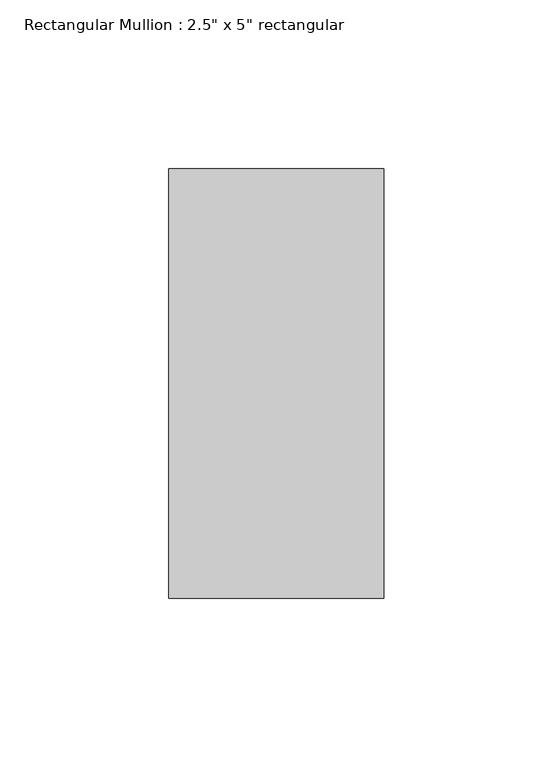
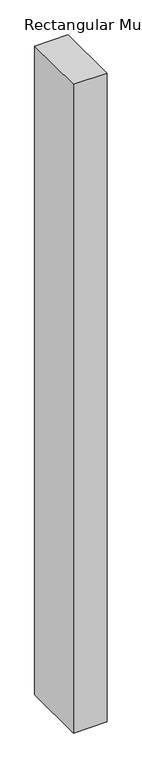
"""IFC4 building model written with IfcOpenShell, lengths in millimetres: member geometry."""

from ifc_helpers import new_model, si_unit, frame, origin, place, context, project, spatial, polyline, outline, extrude, source, transform, mapped, element, save


def member_3e91fb70(model_context):
    return source(origin(), model_context, "Body", "SweptSolid", [
        extrude(outline(polyline([(0.0, 63.5), (0.0, -63.5), (-63.5, -63.5), (-63.5, 63.5), (0.0, 63.5)])), frame((0.0, 0.0, -1298.2581531), z_axis=(0.0, 0.0, 1.0), x_axis=(1.0, 0.0, 0.0)), (0.0, 0.0, 1.0), 1298.2581531),
    ])


if __name__ == "__main__":
    model = new_model("IFC4")
    model_context = context("Model", 3, world=origin())
    ifc_project = project(units=[si_unit("LENGTHUNIT", "METRE", prefix="MILLI")], contexts=[model_context])
    site = spatial("IfcSite", under=ifc_project)
    building = spatial("IfcBuilding", under=site)
    placement = place(None, origin())
    member_shape = member_3e91fb70(model_context)
    element("IfcMember", 1, ObjectType="Rectangular Mullion : 2.5\" x 5\" rectangular", at=placement, inside=building, context=model_context, shape_type="MappedRepresentation", body=[
        mapped(member_shape, transform((0.0, 0.0, 0.0), x_axis=(1.0, 0.0, 0.0), y_axis=(0.0, 1.0, 0.0), z_axis=(0.0, 0.0, 1.0))),
    ])
    save(model, "model.ifc")

# Revit data of these elements
# Type "Rectangular Mullion : 2.5\" x 5\" rectangular"
#   built-in parameter 1007304 = 0.416667 (stored number, unit not read)
#   built-in parameter 1007301 = 0.104167 (stored number, unit not read)
#   built-in parameter 1007300 = 0.104167 (stored number, unit not read)
# Element 1 (IfcMember, "Rectangular Mullion : 2.5\" x 5\" rectangular")
#   Materials on its faces: "Aluminum"
# Materials
#   "Aluminum": class "Metal", colour RGB 247 247 247, transparency 0, Description = "Aluminum 6061", Cost = 0
